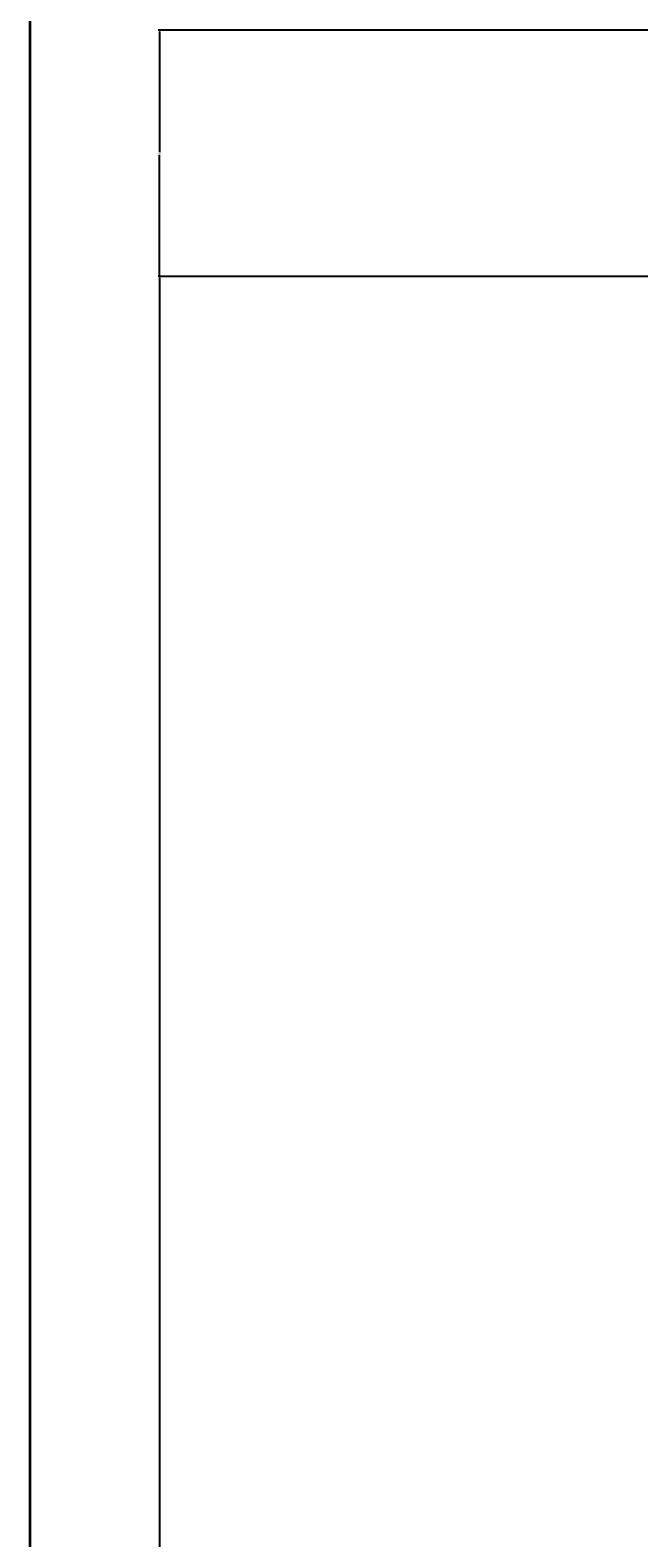
# Model space of a CAD drawing. Units: inches. Extents: x 1885 to 2748, y 783 to 2421.
# Tile 29 of 117: x 1885 to 1969, y 1350 to 1558. Entities that reach past the tile are written whole.
import ezdxf

# ---------------------------------------------------------------- set-up
doc = ezdxf.new("R2010")
doc.units = ezdxf.units.IN
doc.layers.add('A-ANNO-DIMS', color=2, linetype='Continuous', lineweight=18)
doc.layers.add('A-ANNO-TTLB', color=7, linetype='Continuous', lineweight=35)
doc.styles.get("Standard").update_dxf_attribs({"font": 'arial.ttf'})
doc.dimstyles.get("Standard").update_dxf_attribs({"dimtxt": 0.18, "dimasz": 0.18, "dimexe": 0.18, "dimexo": 0.0625, "dimgap": 0.09, "dimtad": 0, "dimtih": 1, "dimtoh": 1, "dimdec": 4, "dimzin": 0, "dimdsep": 46, "dimtxsty": 'Standard', "dimcen": 0.09, "dimadec": 0, "dimazin": 0, "dimtfac": 1, "dimtdec": 4, "dimtofl": 0, "dimtmove": 0, "dimatfit": 3, "dimfxl": 1, "dimtolj": 1, "dimtzin": 0, "dimarcsym": 0})

# ---------------------------------------------------------------- blocks, each defined once
blk = doc.blocks.new('*D45')
at = {"layer": 'A-ANNO-DIMS', "color": 0, "lineweight": -2, "transparency": 16777216}
for p, q in [((1980.71, 1524.01), (1902.84, 1524.01)), ((1903.02, 1523.83), (1903.02, 1290.94)), ((1903.02, 1057.69), (1903.02, 1290.57)), ((1971.21, 1057.51), (1902.84, 1057.51))]:
    blk.add_line(p, q, dxfattribs=at)
at = {"layer": 'A-ANNO-DIMS', "color": 0, "transparency": 16777216}
for points in [[(1902.99, 1523.83), (1903.05, 1523.83), (1903.02, 1524.01)], [(1902.99, 1057.69), (1903.05, 1057.69), (1903.02, 1057.51)]]:
    blk.add_solid(points, dxfattribs=at)
at = {"layer": 'Defpoints', "color": 0, "transparency": 16777216}
for p in [(1903.02, 1524.01), (1980.77, 1524.01), (1971.27, 1057.51)]:
    blk.add_point(p, dxfattribs=at)
at = {"layer": 'A-ANNO-DIMS', "color": 0, "transparency": 16777216, "insert": (1903.02, 1290.76), "char_height": 0.18, "attachment_point": 5}
blk.add_mtext('\\A1;466.5', dxfattribs=at)
blk = doc.blocks.new('*D46')
at = {"layer": 'A-ANNO-DIMS', "color": 0, "lineweight": -2, "transparency": 16777216}
for p, q in [((1980.71, 1558.01), (1902.84, 1558.01)), ((1903.02, 1557.83), (1903.02, 1541.19)), ((1903.02, 1524.19), (1903.02, 1540.82)), ((1980.71, 1524.01), (1902.84, 1524.01))]:
    blk.add_line(p, q, dxfattribs=at)
at = {"layer": 'A-ANNO-DIMS', "color": 0, "transparency": 16777216}
for points in [[(1902.99, 1557.83), (1903.05, 1557.83), (1903.02, 1558.01)], [(1902.99, 1524.19), (1903.05, 1524.19), (1903.02, 1524.01)]]:
    blk.add_solid(points, dxfattribs=at)
at = {"layer": 'Defpoints', "color": 0, "transparency": 16777216}
for p in [(1903.02, 1558.01), (1980.77, 1558.01), (1980.77, 1524.01)]:
    blk.add_point(p, dxfattribs=at)
at = {"layer": 'A-ANNO-DIMS', "color": 0, "transparency": 16777216, "insert": (1903.02, 1541.01), "char_height": 0.18, "attachment_point": 5}
blk.add_mtext('\\A1;34', dxfattribs=at)

msp = doc.modelspace()

# ---------------------------------------------------------------- linework, layer by layer
at = {"layer": 'A-ANNO-TTLB'}
msp.add_lwpolyline([(1885.16, 2409.17), (2748.2, 2409.17), (2748.2, 922.58), (1885.16, 922.58)], close=True, dxfattribs=at)

# ---------------------------------------------------------------- dimensions: what is measured, and where the dimension line sits
at = {"layer": 'A-ANNO-DIMS'}
for base, p1, p2, override, picture, middle in [((1903.02, 1558.01), (1980.77, 1524.01), (1980.77, 1558.01), {"dimdec": 0, "dimlfac": 1, "dimrnd": 0, "dimzin": 0, "dimdsep": 46, "dimlunit": 2}, '*D46', (1903.02, 1541.01)), ((1903.02, 1524.01), (1971.27, 1057.51), (1980.77, 1524.01), {"dimdec": 1, "dimlfac": 1, "dimrnd": 0, "dimzin": 0, "dimdsep": 46, "dimlunit": 2}, '*D45', (1903.02, 1290.76))]:
    dim = msp.add_linear_dim(base=base, p1=p1, p2=p2, angle=90, dimstyle='Standard', override=override, dxfattribs=at)
    dim.commit()
    dim.dimension.update_dxf_attribs({"geometry": picture, "text_midpoint": middle})

doc.saveas('drawing.dxf')
